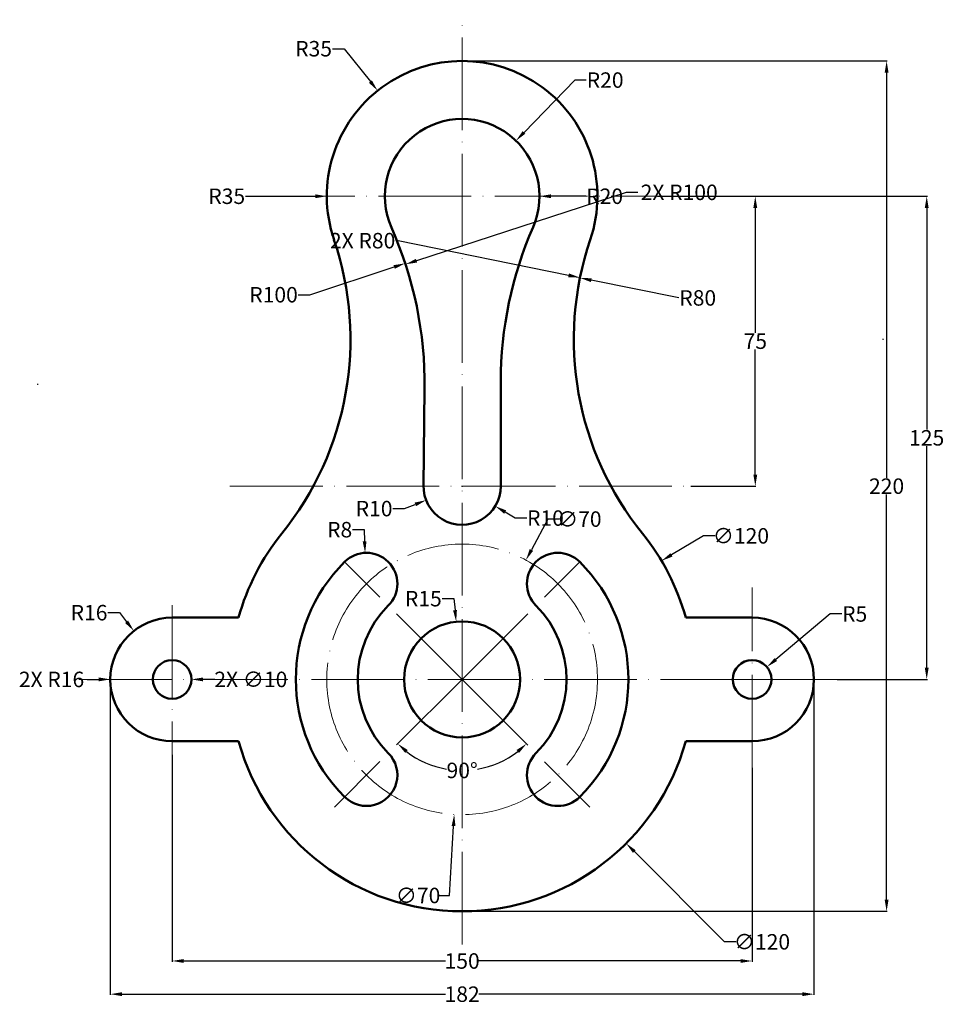
# Model space of a CAD drawing. Units: inches. Extents: x 203 to 442, y 79 to 333.
import ezdxf

# ---------------------------------------------------------------- set-up
doc = ezdxf.new("R2010")
doc.units = ezdxf.units.IN
doc.header["$MEASUREMENT"] = 0
doc.linetypes.add('ACAD_ISO04W100', pattern=[30, 24, -3, 0, -3])
for name, color, linetype, lineweight in [('M-CNTR', 4, 'ACAD_ISO04W100', 18), ('M-DIMS', 2, 'Continuous', 25), ('M-OUTL', 7, 'Continuous', 50)]:
    doc.layers.add(name, color=color, linetype=linetype, lineweight=lineweight)
doc.styles.get("Standard").update_dxf_attribs({"font": 'arial.ttf'})
doc.dimstyles.get("Standard").update_dxf_attribs({"dimtxt": 4, "dimasz": 3, "dimexe": 0.18, "dimexo": 0.0625, "dimgap": 0.09, "dimtad": 0, "dimtih": 1, "dimtoh": 1, "dimdec": 0, "dimzin": 0, "dimdsep": 46, "dimtxsty": 'Standard', "dimcen": 0.09, "dimclrd": 1, "dimclre": 1, "dimadec": 0, "dimazin": 0, "dimtfac": 1, "dimtdec": 0, "dimtofl": 0, "dimtmove": 0, "dimatfit": 3, "dimfxl": 1, "dimtolj": 1, "dimtzin": 0, "dimarcsym": 0})

# ---------------------------------------------------------------- blocks, each defined once
blk = doc.blocks.new('*D1')
at = {"layer": 'Defpoints', "color": 0, "transparency": 16777216}
for p in [(317.35, 162.57), (317.35, 162.57), (311.25, 139.82), (284.31, 129.54), (350.38, 129.54)]:
    blk.add_point(p, dxfattribs=at)
at = {"layer": 'M-DIMS', "color": 0, "lineweight": -2, "transparency": 16777216}
for start, end in [(232.3038, 260.1872), (279.8128, 307.6962)]:
    blk.add_arc((317.35, 162.57), 23.55, start, end, dxfattribs=at)
at = {"layer": 'M-DIMS', "color": 0, "transparency": 16777216}
for points in [[(302.62, 143.56), (303.28, 144.31), (300.69, 145.92)], [(331.42, 144.31), (332.08, 143.56), (334, 145.92)]]:
    blk.add_solid(points, dxfattribs=at)
at = {"layer": 'M-DIMS', "color": 0, "transparency": 16777216, "insert": (317.35, 139.02), "char_height": 4, "attachment_point": 5}
blk.add_mtext('\\A1;90°', dxfattribs=at)
blk = doc.blocks.new('*D2')
at = {"layer": 'Defpoints', "color": 0, "transparency": 16777216}
for p in [(292.25, 195.31), (292.6, 187.32)]:
    blk.add_point(p, dxfattribs=at)
at = {"layer": 'M-DIMS', "color": 0, "lineweight": -2, "transparency": 16777216}
for p, q in [((288.99, 201.31), (291.99, 201.31)), ((291.99, 201.31), (292.12, 198.31)), ((292.51, 187.32), (292.69, 187.32)), ((292.6, 187.23), (292.6, 187.41))]:
    blk.add_line(p, q, dxfattribs=at)
at = {"layer": 'M-DIMS', "color": 0, "transparency": 16777216}
blk.add_solid([(292.62, 198.33), (291.62, 198.29), (292.25, 195.31)], dxfattribs=at)
at = {"layer": 'M-DIMS', "color": 0, "transparency": 16777216, "insert": (285.67, 201.31), "char_height": 4, "attachment_point": 5}
blk.add_mtext('\\A1;R8', dxfattribs=at)
blk = doc.blocks.new('*D3')
at = {"layer": 'Defpoints', "color": 0, "transparency": 16777216}
for p in [(232.43, 175.13), (242.35, 162.57)]:
    blk.add_point(p, dxfattribs=at)
at = {"layer": 'M-DIMS', "color": 0, "lineweight": -2, "transparency": 16777216}
for p, q in [((225.71, 179.84), (228.71, 179.84)), ((228.71, 179.84), (230.57, 177.48)), ((242.26, 162.57), (242.44, 162.57)), ((242.35, 162.48), (242.35, 162.66))]:
    blk.add_line(p, q, dxfattribs=at)
at = {"layer": 'M-DIMS', "color": 0, "transparency": 16777216}
blk.add_solid([(230.96, 177.79), (230.18, 177.17), (232.43, 175.13)], dxfattribs=at)
at = {"layer": 'M-DIMS', "color": 0, "transparency": 16777216, "insert": (220.85, 179.84), "char_height": 4, "attachment_point": 5}
blk.add_mtext('\\A1;R16', dxfattribs=at)
blk = doc.blocks.new('*D4')
at = {"layer": 'Defpoints', "color": 0, "transparency": 16777216}
for p in [(368.91, 193.24), (265.78, 131.9)]:
    blk.add_point(p, dxfattribs=at)
at = {"layer": 'M-DIMS', "color": 0, "lineweight": -2, "transparency": 16777216}
for p, q in [((379.79, 199.71), (371.49, 194.78)), ((382.79, 199.71), (379.79, 199.71)), ((317.26, 162.57), (317.44, 162.57)), ((317.35, 162.48), (317.35, 162.66))]:
    blk.add_line(p, q, dxfattribs=at)
at = {"layer": 'M-DIMS', "color": 0, "transparency": 16777216}
blk.add_solid([(371.24, 195.21), (371.75, 194.35), (368.91, 193.24)], dxfattribs=at)
at = {"layer": 'M-DIMS', "color": 0, "transparency": 16777216, "insert": (389.46, 199.71), "char_height": 4, "attachment_point": 5}
blk.add_mtext('\\A1;∅120', dxfattribs=at)
blk = doc.blocks.new('*D5')
at = {"layer": 'Defpoints', "color": 0, "transparency": 16777216}
for p in [(396.18, 165.78), (392.35, 162.57)]:
    blk.add_point(p, dxfattribs=at)
at = {"layer": 'M-DIMS', "color": 0, "lineweight": -2, "transparency": 16777216}
for p, q in [((412.55, 179.5), (398.48, 167.71)), ((415.55, 179.5), (412.55, 179.5)), ((392.26, 162.57), (392.44, 162.57)), ((392.35, 162.48), (392.35, 162.66))]:
    blk.add_line(p, q, dxfattribs=at)
at = {"layer": 'M-DIMS', "color": 0, "transparency": 16777216}
blk.add_solid([(398.16, 168.09), (398.8, 167.33), (396.18, 165.78)], dxfattribs=at)
at = {"layer": 'M-DIMS', "color": 0, "transparency": 16777216, "insert": (418.88, 179.5), "char_height": 4, "attachment_point": 5}
blk.add_mtext('\\A1;R5', dxfattribs=at)
blk = doc.blocks.new('*D6')
at = {"layer": 'Defpoints', "color": 0, "transparency": 16777216}
for p in [(315.81, 177.49), (317.35, 162.57)]:
    blk.add_point(p, dxfattribs=at)
at = {"layer": 'M-DIMS', "color": 0, "lineweight": -2, "transparency": 16777216}
for p, q in [((312.2, 183.46), (315.2, 183.46)), ((315.2, 183.46), (315.51, 180.48)), ((317.26, 162.57), (317.44, 162.57)), ((317.35, 162.48), (317.35, 162.66))]:
    blk.add_line(p, q, dxfattribs=at)
at = {"layer": 'M-DIMS', "color": 0, "transparency": 16777216}
blk.add_solid([(316, 180.53), (315.01, 180.43), (315.81, 177.49)], dxfattribs=at)
at = {"layer": 'M-DIMS', "color": 0, "transparency": 16777216, "insert": (307.31, 183.46), "char_height": 4, "attachment_point": 5}
blk.add_mtext('\\A1;R15', dxfattribs=at)
blk = doc.blocks.new('*D7')
at = {"layer": 'Defpoints', "color": 0, "transparency": 16777216}
for p in [(333.85, 193.43), (300.84, 131.71)]:
    blk.add_point(p, dxfattribs=at)
at = {"layer": 'M-DIMS', "color": 0, "lineweight": -2, "transparency": 16777216}
for p, q in [((339.53, 204.04), (335.27, 196.08)), ((342.53, 204.04), (339.53, 204.04)), ((317.26, 162.57), (317.44, 162.57)), ((317.35, 162.48), (317.35, 162.66))]:
    blk.add_line(p, q, dxfattribs=at)
at = {"layer": 'M-DIMS', "color": 0, "transparency": 16777216}
blk.add_solid([(334.83, 196.32), (335.71, 195.84), (333.85, 193.43)], dxfattribs=at)
at = {"layer": 'M-DIMS', "color": 0, "transparency": 16777216, "insert": (347.65, 204.04), "char_height": 4, "attachment_point": 5}
blk.add_mtext('\\A1;∅70', dxfattribs=at)
blk = doc.blocks.new('*D8')
at = {"layer": 'Defpoints', "color": 0, "transparency": 16777216}
for p in [(242.35, 143.13), (392.35, 139.75), (392.35, 89.72)]:
    blk.add_point(p, dxfattribs=at)
at = {"layer": 'M-DIMS', "color": 0, "lineweight": -2, "transparency": 16777216}
for p, q in [((242.35, 143.06), (242.35, 89.54)), ((392.35, 139.69), (392.35, 89.54)), ((245.35, 89.72), (313.03, 89.72)), ((389.35, 89.72), (321.66, 89.72))]:
    blk.add_line(p, q, dxfattribs=at)
at = {"layer": 'M-DIMS', "color": 0, "transparency": 16777216}
for points in [[(245.35, 90.22), (245.35, 89.22), (242.35, 89.72)], [(389.35, 90.22), (389.35, 89.22), (392.35, 89.72)]]:
    blk.add_solid(points, dxfattribs=at)
at = {"layer": 'M-DIMS', "color": 0, "transparency": 16777216, "insert": (317.35, 89.72), "char_height": 4, "attachment_point": 5}
blk.add_mtext('\\A1;150', dxfattribs=at)
blk = doc.blocks.new('*D9')
at = {"layer": 'Defpoints', "color": 0, "transparency": 16777216}
for p in [(317.35, 212.57), (308.03, 208.94)]:
    blk.add_point(p, dxfattribs=at)
at = {"layer": 'M-DIMS', "color": 0, "lineweight": -2, "transparency": 16777216}
for p, q in [((317.26, 212.57), (317.44, 212.57)), ((317.35, 212.48), (317.35, 212.66)), ((299.44, 206.76), (302.44, 206.76)), ((302.44, 206.76), (305.24, 207.85))]:
    blk.add_line(p, q, dxfattribs=at)
at = {"layer": 'M-DIMS', "color": 0, "transparency": 16777216}
blk.add_solid([(305.05, 208.31), (305.42, 207.38), (308.03, 208.94)], dxfattribs=at)
at = {"layer": 'M-DIMS', "color": 0, "transparency": 16777216, "insert": (294.58, 206.76), "char_height": 4, "attachment_point": 5}
blk.add_mtext('\\A1;R10', dxfattribs=at)
blk = doc.blocks.new('*D10')
at = {"layer": 'Defpoints', "color": 0, "transparency": 16777216}
for p in [(347.82, 266.45), (426.23, 250.57)]:
    blk.add_point(p, dxfattribs=at)
at = {"layer": 'M-DIMS', "color": 0, "lineweight": -2, "transparency": 16777216}
blk.add_line((373.41, 261.27), (350.76, 265.85), dxfattribs=at)
at = {"layer": 'M-DIMS', "color": 0, "transparency": 16777216}
blk.add_solid([(350.86, 266.34), (350.66, 265.36), (347.82, 266.45)], dxfattribs=at)
at = {"layer": 'M-DIMS', "color": 0, "transparency": 16777216, "insert": (378.28, 261.27), "char_height": 4, "attachment_point": 5}
blk.add_mtext('\\A1;R80', dxfattribs=at)
blk = doc.blocks.new('*D11')
at = {"layer": 'Defpoints', "color": 0, "transparency": 16777216}
for p in [(367.85, 287.57), (376.4, 212.57), (393.17, 212.57)]:
    blk.add_point(p, dxfattribs=at)
at = {"layer": 'M-DIMS', "color": 0, "lineweight": -2, "transparency": 16777216}
for p, q in [((367.91, 287.57), (393.35, 287.57)), ((393.17, 284.57), (393.17, 252.2)), ((393.17, 215.57), (393.17, 247.95)), ((376.46, 212.57), (393.35, 212.57))]:
    blk.add_line(p, q, dxfattribs=at)
at = {"layer": 'M-DIMS', "color": 0, "transparency": 16777216}
for points in [[(392.67, 284.57), (393.67, 284.57), (393.17, 287.57)], [(392.67, 215.57), (393.67, 215.57), (393.17, 212.57)]]:
    blk.add_solid(points, dxfattribs=at)
at = {"layer": 'M-DIMS', "color": 0, "transparency": 16777216, "insert": (393.17, 250.07), "char_height": 4, "attachment_point": 5}
blk.add_mtext('\\A1;75', dxfattribs=at)
blk = doc.blocks.new('*D12')
at = {"layer": 'Defpoints', "color": 0, "transparency": 16777216}
for p in [(367.85, 287.57), (414.31, 162.57), (437.51, 162.57)]:
    blk.add_point(p, dxfattribs=at)
at = {"layer": 'M-DIMS', "color": 0, "lineweight": -2, "transparency": 16777216}
for p, q in [((367.91, 287.57), (437.69, 287.57)), ((437.51, 284.57), (437.51, 227.2)), ((437.51, 165.57), (437.51, 222.94)), ((414.37, 162.57), (437.69, 162.57))]:
    blk.add_line(p, q, dxfattribs=at)
at = {"layer": 'M-DIMS', "color": 0, "transparency": 16777216}
for points in [[(437.01, 284.57), (438.01, 284.57), (437.51, 287.57)], [(437.01, 165.57), (438.01, 165.57), (437.51, 162.57)]]:
    blk.add_solid(points, dxfattribs=at)
at = {"layer": 'M-DIMS', "color": 0, "transparency": 16777216, "insert": (437.51, 225.07), "char_height": 4, "attachment_point": 5}
blk.add_mtext('\\A1;125', dxfattribs=at)
blk = doc.blocks.new('*D13')
at = {"layer": 'Defpoints', "color": 0, "transparency": 16777216}
for p in [(302.63, 270.21), (207.64, 238.94)]:
    blk.add_point(p, dxfattribs=at)
at = {"layer": 'M-DIMS', "color": 0, "lineweight": -2, "transparency": 16777216}
for p, q in [((277.98, 262.09), (299.78, 269.27)), ((274.98, 262.09), (277.98, 262.09))]:
    blk.add_line(p, q, dxfattribs=at)
at = {"layer": 'M-DIMS', "color": 0, "transparency": 16777216}
blk.add_solid([(299.62, 269.74), (299.94, 268.8), (302.63, 270.21)], dxfattribs=at)
at = {"layer": 'M-DIMS', "color": 0, "transparency": 16777216, "insert": (268.57, 262.09), "char_height": 4, "attachment_point": 5}
blk.add_mtext('\\A1;R100', dxfattribs=at)
blk = doc.blocks.new('*D14')
at = {"layer": 'Defpoints', "color": 0, "transparency": 16777216}
for p in [(295.48, 314.9), (317.35, 287.57)]:
    blk.add_point(p, dxfattribs=at)
at = {"layer": 'M-DIMS', "color": 0, "lineweight": -2, "transparency": 16777216}
for p, q in [((283.81, 325.74), (286.81, 325.74)), ((286.81, 325.74), (293.61, 317.24)), ((317.26, 287.57), (317.44, 287.57)), ((317.35, 287.48), (317.35, 287.66))]:
    blk.add_line(p, q, dxfattribs=at)
at = {"layer": 'M-DIMS', "color": 0, "transparency": 16777216}
blk.add_solid([(294, 317.56), (293.22, 316.93), (295.48, 314.9)], dxfattribs=at)
at = {"layer": 'M-DIMS', "color": 0, "transparency": 16777216, "insert": (278.93, 325.74), "char_height": 4, "attachment_point": 5}
blk.add_mtext('\\A1;R35', dxfattribs=at)
blk = doc.blocks.new('*D15')
at = {"layer": 'Defpoints', "color": 0, "transparency": 16777216}
for p in [(331.27, 301.93), (317.35, 287.57)]:
    blk.add_point(p, dxfattribs=at)
at = {"layer": 'M-DIMS', "color": 0, "lineweight": -2, "transparency": 16777216}
for p, q in [((346.47, 317.62), (333.36, 304.09)), ((349.47, 317.62), (346.47, 317.62)), ((317.26, 287.57), (317.44, 287.57)), ((317.35, 287.48), (317.35, 287.66))]:
    blk.add_line(p, q, dxfattribs=at)
at = {"layer": 'M-DIMS', "color": 0, "transparency": 16777216}
blk.add_solid([(333, 304.43), (333.71, 303.74), (331.27, 301.93)], dxfattribs=at)
at = {"layer": 'M-DIMS', "color": 0, "transparency": 16777216, "insert": (354.34, 317.62), "char_height": 4, "attachment_point": 5}
blk.add_mtext('\\A1;R20', dxfattribs=at)
blk = doc.blocks.new('LINK-ARCUATE-SLOT')
for centre, radius, start, end in [((24.75, 24.75), 8, 45, 225), ((0, 0), 43, 315, 45), ((0, 0), 27, 315, 45), ((24.75, -24.75), 8, 135, 315)]:
    blk.add_arc(centre, radius, start, end)
blk = doc.blocks.new('LINK-MOUNTING-EAR')
for p, q in [((0, 16), (-17.17, 16)), ((0, -16), (-17.17, -16))]:
    blk.add_line(p, q)
blk.add_circle((0, 0), 5)
blk.add_arc((0, 0), 16, 270, 90)
blk = doc.blocks.new('*D18')
at = {"layer": 'Defpoints', "color": 0, "transparency": 16777216}
for p in [(317.35, 322.57), (427.13, 322.57), (317.35, 102.57)]:
    blk.add_point(p, dxfattribs=at)
at = {"layer": 'M-DIMS', "color": 1, "lineweight": -2, "transparency": 16777216}
for p, q in [((317.41, 322.57), (427.31, 322.57)), ((427.13, 319.57), (427.13, 214.7)), ((427.13, 105.57), (427.13, 210.44)), ((317.41, 102.57), (427.31, 102.57))]:
    blk.add_line(p, q, dxfattribs=at)
at = {"layer": 'M-DIMS', "color": 1, "transparency": 16777216}
for points in [[(426.63, 319.57), (427.63, 319.57), (427.13, 322.57)], [(426.63, 105.57), (427.63, 105.57), (427.13, 102.57)]]:
    blk.add_solid(points, dxfattribs=at)
at = {"layer": 'M-DIMS', "color": 0, "transparency": 16777216, "insert": (427.13, 212.57), "char_height": 4, "attachment_point": 5}
blk.add_mtext('\\A1;220', dxfattribs=at)
blk = doc.blocks.new('*D19')
at = {"layer": 'Defpoints', "color": 0, "transparency": 16777216}
for p in [(226.35, 162.57), (408.35, 162.57), (408.35, 81.14)]:
    blk.add_point(p, dxfattribs=at)
at = {"layer": 'M-DIMS', "color": 1, "lineweight": -2, "transparency": 16777216}
for p, q in [((226.35, 162.51), (226.35, 80.96)), ((408.35, 162.51), (408.35, 80.96)), ((229.35, 81.14), (313.05, 81.14)), ((405.35, 81.14), (321.65, 81.14))]:
    blk.add_line(p, q, dxfattribs=at)
at = {"layer": 'M-DIMS', "color": 1, "transparency": 16777216}
for points in [[(229.35, 81.64), (229.35, 80.64), (226.35, 81.14)], [(405.35, 81.64), (405.35, 80.64), (408.35, 81.14)]]:
    blk.add_solid(points, dxfattribs=at)
at = {"layer": 'M-DIMS', "color": 0, "transparency": 16777216, "insert": (317.35, 81.14), "char_height": 4, "attachment_point": 5}
blk.add_mtext('\\A1;182', dxfattribs=at)
blk = doc.blocks.new('*D20')
at = {"layer": 'Defpoints', "color": 0, "transparency": 16777216}
for p in [(282.35, 287.57), (317.35, 287.57)]:
    blk.add_point(p, dxfattribs=at)
at = {"layer": 'M-DIMS', "color": 1, "lineweight": -2, "transparency": 16777216}
for p, q in [((261.35, 287.57), (279.35, 287.57)), ((317.26, 287.57), (317.44, 287.57)), ((317.35, 287.48), (317.35, 287.66))]:
    blk.add_line(p, q, dxfattribs=at)
at = {"layer": 'M-DIMS', "color": 1, "transparency": 16777216}
blk.add_solid([(279.35, 288.07), (279.35, 287.07), (282.35, 287.57)], dxfattribs=at)
at = {"layer": 'M-DIMS', "color": 0, "transparency": 16777216, "insert": (256.46, 287.57), "char_height": 4, "attachment_point": 5}
blk.add_mtext('\\A1;R35', dxfattribs=at)
blk = doc.blocks.new('*D21')
at = {"layer": 'Defpoints', "color": 0, "transparency": 16777216}
for p in [(317.35, 287.57), (337.35, 287.57)]:
    blk.add_point(p, dxfattribs=at)
at = {"layer": 'M-DIMS', "color": 1, "lineweight": -2, "transparency": 16777216}
for p, q in [((317.26, 287.57), (317.44, 287.57)), ((317.35, 287.48), (317.35, 287.66)), ((349.35, 287.57), (340.35, 287.57))]:
    blk.add_line(p, q, dxfattribs=at)
at = {"layer": 'M-DIMS', "color": 1, "transparency": 16777216}
blk.add_solid([(340.35, 288.07), (340.35, 287.07), (337.35, 287.57)], dxfattribs=at)
at = {"layer": 'M-DIMS', "color": 0, "transparency": 16777216, "insert": (354.21, 287.57), "char_height": 4, "attachment_point": 5}
blk.add_mtext('\\A1;R20', dxfattribs=at)
blk = doc.blocks.new('*D22')
at = {"layer": 'Defpoints', "color": 0, "transparency": 16777216}
for p in [(347.84, 266.51), (426.23, 250.57)]:
    blk.add_point(p, dxfattribs=at)
at = {"layer": 'M-DIMS', "color": 1, "lineweight": -2, "transparency": 16777216}
for p, q in [((300.8, 276.08), (344.9, 267.11)), ((426.14, 250.57), (426.32, 250.57)), ((426.23, 250.48), (426.23, 250.66))]:
    blk.add_line(p, q, dxfattribs=at)
at = {"layer": 'M-DIMS', "color": 1, "transparency": 16777216}
blk.add_solid([(345, 267.6), (344.8, 266.62), (347.84, 266.51)], dxfattribs=at)
at = {"layer": 'M-DIMS', "color": 0, "transparency": 16777216, "insert": (291.61, 276.08), "char_height": 4, "attachment_point": 5}
blk.add_mtext('\\A1;2X R80', dxfattribs=at)
blk = doc.blocks.new('*D23')
at = {"layer": 'Defpoints', "color": 0, "transparency": 16777216}
for p in [(302.71, 269.97), (207.64, 238.94)]:
    blk.add_point(p, dxfattribs=at)
at = {"layer": 'M-DIMS', "color": 1, "lineweight": -2, "transparency": 16777216}
for p, q in [((359.75, 288.58), (305.56, 270.9)), ((362.75, 288.58), (359.75, 288.58)), ((207.55, 238.94), (207.73, 238.94)), ((207.64, 238.85), (207.64, 239.03))]:
    blk.add_line(p, q, dxfattribs=at)
at = {"layer": 'M-DIMS', "color": 1, "transparency": 16777216}
blk.add_solid([(305.4, 271.37), (305.71, 270.42), (302.71, 269.97)], dxfattribs=at)
at = {"layer": 'M-DIMS', "color": 0, "transparency": 16777216, "insert": (373.49, 288.58), "char_height": 4, "attachment_point": 5}
blk.add_mtext('\\A1;2X R100', dxfattribs=at)
blk = doc.blocks.new('*D24')
at = {"layer": 'Defpoints', "color": 0, "transparency": 16777216}
for p in [(317.35, 212.57), (325.91, 207.41)]:
    blk.add_point(p, dxfattribs=at)
at = {"layer": 'M-DIMS', "color": 1, "lineweight": -2, "transparency": 16777216}
for p, q in [((317.26, 212.57), (317.44, 212.57)), ((317.35, 212.48), (317.35, 212.66)), ((331.05, 204.31), (328.48, 205.86)), ((334.05, 204.31), (331.05, 204.31))]:
    blk.add_line(p, q, dxfattribs=at)
at = {"layer": 'M-DIMS', "color": 1, "transparency": 16777216}
blk.add_solid([(328.74, 206.29), (328.22, 205.43), (325.91, 207.41)], dxfattribs=at)
at = {"layer": 'M-DIMS', "color": 0, "transparency": 16777216, "insert": (338.91, 204.31), "char_height": 4, "attachment_point": 5}
blk.add_mtext('\\A1;R10', dxfattribs=at)
blk = doc.blocks.new('*D25')
at = {"layer": 'Defpoints', "color": 0, "transparency": 16777216}
for p in [(274.92, 205), (359.77, 120.14)]:
    blk.add_point(p, dxfattribs=at)
at = {"layer": 'M-DIMS', "color": 1, "lineweight": -2, "transparency": 16777216}
for p, q in [((317.26, 162.57), (317.44, 162.57)), ((317.35, 162.48), (317.35, 162.66)), ((385.22, 94.68), (361.89, 118.02)), ((388.22, 94.68), (385.22, 94.68))]:
    blk.add_line(p, q, dxfattribs=at)
at = {"layer": 'M-DIMS', "color": 1, "transparency": 16777216}
blk.add_solid([(362.24, 118.37), (361.54, 117.67), (359.77, 120.14)], dxfattribs=at)
at = {"layer": 'M-DIMS', "color": 0, "transparency": 16777216, "insert": (394.9, 94.68), "char_height": 4, "attachment_point": 5}
blk.add_mtext('\\A1;∅120', dxfattribs=at)
blk = doc.blocks.new('*D26')
at = {"layer": 'Defpoints', "color": 0, "transparency": 16777216}
for p in [(226.35, 162.57), (242.35, 162.57)]:
    blk.add_point(p, dxfattribs=at)
at = {"layer": 'M-DIMS', "color": 1, "lineweight": -2, "transparency": 16777216}
for p, q in [((220.35, 162.57), (223.35, 162.57)), ((242.26, 162.57), (242.44, 162.57)), ((242.35, 162.48), (242.35, 162.66))]:
    blk.add_line(p, q, dxfattribs=at)
at = {"layer": 'M-DIMS', "color": 1, "transparency": 16777216}
blk.add_solid([(223.35, 163.07), (223.35, 162.07), (226.35, 162.57)], dxfattribs=at)
at = {"layer": 'M-DIMS', "color": 0, "transparency": 16777216, "insert": (211.15, 162.57), "char_height": 4, "attachment_point": 5}
blk.add_mtext('\\A1;2X R16', dxfattribs=at)
blk = doc.blocks.new('*D27')
at = {"layer": 'Defpoints', "color": 0, "transparency": 16777216}
for p in [(237.35, 162.57), (247.35, 162.57)]:
    blk.add_point(p, dxfattribs=at)
at = {"layer": 'M-DIMS', "color": 1, "lineweight": -2, "transparency": 16777216}
for p, q in [((242.26, 162.57), (242.44, 162.57)), ((242.35, 162.48), (242.35, 162.66)), ((253.35, 162.57), (250.35, 162.57))]:
    blk.add_line(p, q, dxfattribs=at)
at = {"layer": 'M-DIMS', "color": 1, "transparency": 16777216}
blk.add_solid([(250.35, 163.07), (250.35, 162.07), (247.35, 162.57)], dxfattribs=at)
at = {"layer": 'M-DIMS', "color": 0, "transparency": 16777216, "insert": (262.7, 162.57), "char_height": 4, "attachment_point": 5}
blk.add_mtext('\\A1;2X ∅10', dxfattribs=at)
blk = doc.blocks.new('*D28')
at = {"layer": 'Defpoints', "color": 0, "transparency": 16777216}
for p in [(319.39, 197.51), (315.3, 127.63)]:
    blk.add_point(p, dxfattribs=at)
at = {"layer": 'M-DIMS', "color": 1, "lineweight": -2, "transparency": 16777216}
for p, q in [((317.26, 162.57), (317.44, 162.57)), ((317.35, 162.48), (317.35, 162.66)), ((314.07, 106.67), (315.12, 124.64)), ((311.07, 106.67), (314.07, 106.67))]:
    blk.add_line(p, q, dxfattribs=at)
at = {"layer": 'M-DIMS', "color": 1, "transparency": 16777216}
blk.add_solid([(314.63, 124.67), (315.62, 124.61), (315.3, 127.63)], dxfattribs=at)
at = {"layer": 'M-DIMS', "color": 0, "transparency": 16777216, "insert": (305.95, 106.67), "char_height": 4, "attachment_point": 5}
blk.add_mtext('\\A1;∅70', dxfattribs=at)

msp = doc.modelspace()

# ---------------------------------------------------------------- linework, layer by layer
at = {"layer": 'M-CNTR'}
for p, q in [((317.35, 93.96), (317.35, 333.25)), ((265.58, 287.57), (367.85, 287.57)), ((257.3, 212.57), (376.4, 212.57)), ((317.35, 162.57), (286.94, 192.98)), ((317.35, 162.57), (347.75, 192.98)), ((392.35, 139.75), (392.35, 186.39)), ((242.35, 181.76), (242.35, 143.13)), ((317.35, 162.57), (284.31, 129.54)), ((317.35, 162.57), (350.38, 129.54))]:
    msp.add_line(p, q, dxfattribs=at)
msp.add_lwpolyline([(218.17, 162.57), (392.35, 162.57), (414.31, 162.57)], dxfattribs=at)
msp.add_circle((317.35, 162.57), 35, dxfattribs=at)
at = {"layer": 'M-OUTL'}
for p, q in [((327.35, 212.57), (327.35, 239.61)), ((307.35, 212.57), (307.64, 237.79))]:
    msp.add_line(p, q, dxfattribs=at)
msp.add_circle((317.35, 162.57), 15, dxfattribs=at)
for centre, radius, start, end in [((317.35, 287.57), 35, 341.2319, 198.7681), ((317.35, 287.57), 20, 336.4435, 203.9081), ((207.64, 238.94), 100, 359.3416, 23.9081), ((427.35, 239.61), 100, 156.4435, 180), ((208.46, 250.57), 80, 321.0552, 18.7681), ((426.23, 250.57), 80, 161.2319, 218.9448), ((317.35, 212.57), 10, 178.6833, 0), ((317.35, 162.57), 60, 141.0552, 164.534), ((317.35, 162.57), 60, 15.466, 38.9448), ((317.35, 162.57), 60, 195.466, 344.534)]:
    msp.add_arc(centre, radius, start, end, dxfattribs=at)

# ---------------------------------------------------------------- block references
at = {"layer": 'M-OUTL', "rotation": 180}
for name, p in [('LINK-ARCUATE-SLOT', (317.35, 162.57)), ('LINK-MOUNTING-EAR', (242.35, 162.57))]:
    msp.add_blockref(name, p, dxfattribs=at)
at = {"layer": 'M-OUTL'}
for name, p in [('LINK-ARCUATE-SLOT', (317.35, 162.57)), ('LINK-MOUNTING-EAR', (392.35, 162.57))]:
    msp.add_blockref(name, p, dxfattribs=at)

# ---------------------------------------------------------------- dimensions: what is measured, and where the dimension line sits
at = {"layer": 'M-DIMS'}
for center, mpoint, override, picture, middle in [((317.35, 287.57), (295.48, 314.9), {"dimclrd": 0, "dimclre": 0, "dimclrt": 0}, '*D14', (278.93, 325.74)), ((317.35, 287.57), (331.27, 301.93), {"dimclrd": 0, "dimclre": 0, "dimclrt": 0}, '*D15', (354.34, 317.62)), ((317.35, 287.57), (282.35, 287.57), {"dimdec": 0, "dimlfac": 1, "dimrnd": 0, "dimzin": 0, "dimdsep": 46, "dimlunit": 2}, '*D20', (261.35, 287.57)), ((317.35, 287.57), (337.35, 287.57), {"dimdec": 0, "dimlfac": 1, "dimrnd": 0, "dimzin": 0, "dimdsep": 46, "dimlunit": 2}, '*D21', (349.35, 287.57)), ((207.64, 238.94), (302.63, 270.21), {"dimclrd": 0, "dimclre": 0, "dimclrt": 0}, '*D13', (268.57, 262.09)), ((426.23, 250.57), (347.82, 266.45), {"dimclrd": 0, "dimclre": 0, "dimclrt": 0}, '*D10', (373.41, 261.27)), ((317.35, 212.57), (325.91, 207.41), {"dimdec": 0, "dimlfac": 1, "dimrnd": 0, "dimzin": 0, "dimdsep": 46, "dimlunit": 2}, '*D24', (338.91, 204.31)), ((392.35, 162.57), (396.18, 165.78), {"dimclrd": 0, "dimclre": 0, "dimclrt": 0}, '*D5', (418.88, 179.5))]:
    dim = msp.add_radius_dim(center=center, mpoint=mpoint, dimstyle='Standard', override=override, dxfattribs=at)
    dim.commit()
    dim.dimension.update_dxf_attribs({"geometry": picture, "text_midpoint": middle, "dimtype": 164})
for base, p1, p2, override, picture, middle in [((427.13, 322.57), (317.35, 102.57), (317.35, 322.57), {"dimdec": 0, "dimlfac": 1, "dimrnd": 0, "dimzin": 0, "dimdsep": 46, "dimlunit": 2}, '*D18', (427.13, 212.57)), ((393.17, 212.57), (367.85, 287.57), (376.4, 212.57), {"dimclrd": 0, "dimclre": 0, "dimclrt": 0}, '*D11', (393.17, 250.07)), ((437.51, 162.57), (367.85, 287.57), (414.31, 162.57), {"dimclrd": 0, "dimclre": 0, "dimclrt": 0}, '*D12', (437.51, 225.07))]:
    dim = msp.add_linear_dim(base=base, p1=p1, p2=p2, angle=90, dimstyle='Standard', override=override, dxfattribs=at)
    dim.commit()
    dim.dimension.update_dxf_attribs({"geometry": picture, "text_midpoint": middle})
for center, mpoint, picture, middle in [((207.64, 238.94), (302.71, 269.97), '*D23', (373.49, 288.58)), ((426.23, 250.57), (347.84, 266.51), '*D22', (300.8, 276.08))]:
    dim = msp.add_radius_dim(center=center, mpoint=mpoint, text='2X <>', dimstyle='Standard', override={"dimdec": 0, "dimlfac": 1, "dimrnd": 0, "dimzin": 0, "dimdsep": 46, "dimlunit": 2}, dxfattribs=at)
    dim.commit()
    dim.dimension.update_dxf_attribs({"geometry": picture, "text_midpoint": middle, "dimtype": 164})
for center, mpoint, picture, middle in [((317.35, 212.57), (308.03, 208.94), '*D9', (294.58, 206.76)), ((292.6, 187.32), (292.25, 195.31), '*D2', (285.67, 201.31)), ((317.35, 162.57), (315.81, 177.49), '*D6', (307.31, 183.46)), ((242.35, 162.57), (232.43, 175.13), '*D3', (220.85, 179.84))]:
    dim = msp.add_radius_dim(center=center, mpoint=mpoint, dimstyle='Standard', override={"dimclrd": 0, "dimclre": 0, "dimclrt": 0}, dxfattribs=at)
    dim.commit()
    dim.dimension.update_dxf_attribs({"geometry": picture, "text_midpoint": middle})
for p1, p2, override, picture, middle in [((300.84, 131.71), (333.85, 193.43), {"dimclrd": 0, "dimclre": 0, "dimclrt": 0}, '*D7', (347.65, 204.04)), ((274.92, 205), (359.77, 120.14), {"dimdec": 0, "dimlfac": 1, "dimrnd": 0, "dimzin": 0, "dimdsep": 46, "dimlunit": 2}, '*D25', (394.9, 94.68)), ((265.78, 131.9), (368.91, 193.24), {"dimclrd": 0, "dimclre": 0, "dimclrt": 0}, '*D4', (389.46, 199.71)), ((319.39, 197.51), (315.3, 127.63), {"dimdec": 0, "dimlfac": 1, "dimrnd": 0, "dimzin": 0, "dimdsep": 46, "dimlunit": 2}, '*D28', (305.95, 106.67))]:
    dim = msp.add_diameter_dim_2p(p1=p1, p2=p2, dimstyle='Standard', override=override, dxfattribs=at)
    dim.commit()
    dim.dimension.update_dxf_attribs({"geometry": picture, "text_midpoint": middle, "dimtype": 163})
dim = msp.add_radius_dim(center=(242.35, 162.57), mpoint=(226.35, 162.57), text='2X <>', dimstyle='Standard', override={"dimdec": 0, "dimlfac": 1, "dimrnd": 0, "dimzin": 0, "dimdsep": 46, "dimlunit": 2}, dxfattribs=at)
dim.commit()
dim.dimension.update_dxf_attribs({"geometry": '*D26', "text_midpoint": (211.15, 162.57)})
dim = msp.add_diameter_dim_2p(p1=(237.35, 162.57), p2=(247.35, 162.57), text='2X <>', dimstyle='Standard', override={"dimdec": 0, "dimlfac": 1, "dimrnd": 0, "dimzin": 0, "dimdsep": 46, "dimlunit": 2}, dxfattribs=at)
dim.commit()
dim.dimension.update_dxf_attribs({"geometry": '*D27', "text_midpoint": (253.35, 162.57), "dimtype": 163})
for base, p1, p2, override, picture, middle in [((408.35, 81.14), (226.35, 162.57), (408.35, 162.57), {"dimdec": 0, "dimlfac": 1, "dimrnd": 0, "dimzin": 0, "dimdsep": 46, "dimlunit": 2}, '*D19', (317.35, 81.14)), ((392.35, 89.72), (242.35, 143.13), (392.35, 139.75), {"dimclrd": 0, "dimclre": 0, "dimclrt": 0}, '*D8', (317.35, 89.72))]:
    dim = msp.add_linear_dim(base=base, p1=p1, p2=p2, dimstyle='Standard', override=override, dxfattribs=at)
    dim.commit()
    dim.dimension.update_dxf_attribs({"geometry": picture, "text_midpoint": middle})
dim = msp.add_angular_dim_2l(base=(311.25, 139.82), line1=((317.35, 162.57), (350.38, 129.54)), line2=((317.35, 162.57), (284.31, 129.54)), dimstyle='Standard', override={"dimclrd": 0, "dimclre": 0, "dimclrt": 0}, dxfattribs=at)
dim.commit()
dim.dimension.update_dxf_attribs({"geometry": '*D1', "text_midpoint": (317.35, 139.02), "dimtype": 162})

doc.saveas('drawing.dxf')
